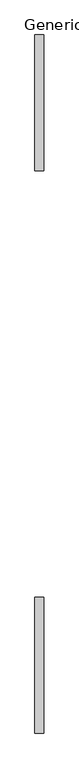
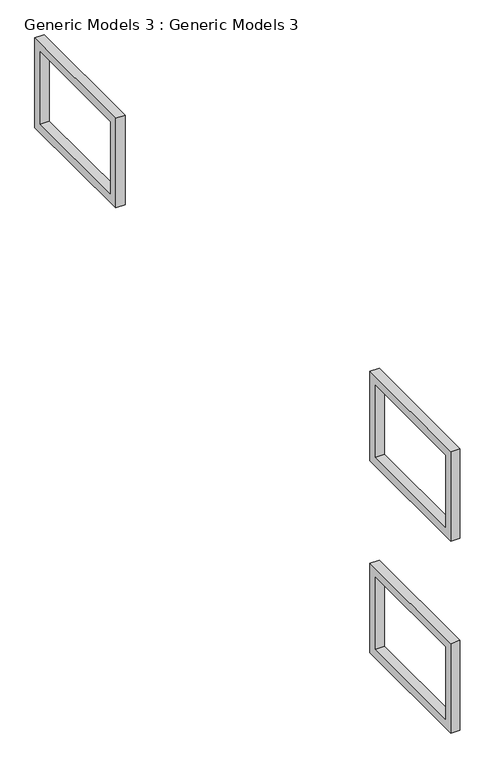
"""IFC4 building model written with IfcOpenShell, lengths in millimetres: proxy geometry, Generic Models 3 : Generic Models 3."""

from ifc_helpers import new_model, si_unit, frame, origin, place, context, project, spatial, polyline, outline, extrude, source, transform, mapped, element, save


def generic_models_3_generic_models_3_62885dc4(model_context):
    return source(origin(), model_context, "Body", "SweptSolid", [
        extrude(outline(polyline([(-2572.1938352, 5765.2), (-257.3938352, 5765.2), (-257.3938352, 4200.4), (-2572.1938352, 4200.4), (-2572.1938352, 5765.2)]), holes=[polyline([(-2419.7938352, 5612.8), (-2419.7938352, 4352.8), (-409.7938352, 4352.8), (-409.7938352, 5612.8), (-2419.7938352, 5612.8)])]), frame((-6909.0474631, 0.0, 0.0), z_axis=(1.0, 0.0, 0.0), x_axis=(0.0, 1.0, 0.0)), (0.0, 0.0, 1.0), 152.4),
        extrude(outline(polyline([(-2572.1938352, 2412.4), (-257.3938352, 2412.4), (-257.3938352, 847.6), (-2572.1938352, 847.6), (-2572.1938352, 2412.4)]), holes=[polyline([(-2419.7938352, 2260.0), (-2419.7938352, 1000.0), (-409.7938352, 1000.0), (-409.7938352, 2260.0), (-2419.7938352, 2260.0)])]), frame((-6909.0474631, 0.0, 0.0), z_axis=(1.0, 0.0, 0.0), x_axis=(0.0, 1.0, 0.0)), (0.0, 0.0, 1.0), 152.4),
        extrude(outline(polyline([(7029.0061648, 5765.2), (9343.8061648, 5765.2), (9343.8061648, 4200.4), (7029.0061648, 4200.4), (7029.0061648, 5765.2)]), holes=[polyline([(7181.4061648, 5612.8), (7181.4061648, 4352.8), (9191.4061648, 4352.8), (9191.4061648, 5612.8), (7181.4061648, 5612.8)])]), frame((-6909.0474631, 0.0, 0.0), z_axis=(1.0, 0.0, 0.0), x_axis=(0.0, 1.0, 0.0)), (0.0, 0.0, 1.0), 152.4),
    ])


if __name__ == "__main__":
    model = new_model("IFC4")
    model_context = context("Model", 3, world=origin())
    ifc_project = project(units=[si_unit("LENGTHUNIT", "METRE", prefix="MILLI")], contexts=[model_context])
    site = spatial("IfcSite", under=ifc_project)
    building = spatial("IfcBuilding", under=site)
    placement = place(None, origin())
    generic_models_3_generic_models_3_shape = generic_models_3_generic_models_3_62885dc4(model_context)
    element("IfcBuildingElementProxy", 1, Name="Generic Models 3 : Generic Models 3", ObjectType="Generic Models 3 : Generic Models 3", at=placement, inside=building, context=model_context, shape_type="MappedRepresentation", body=[
        mapped(generic_models_3_generic_models_3_shape, transform((0.0, 0.0, 0.0), x_axis=(1.0, 0.0, 0.0), y_axis=(0.0, 1.0, 0.0), z_axis=(0.0, 0.0, 1.0))),
    ])
    save(model, "model.ifc")

# Revit data of these elements
# Element 1 (IfcBuildingElementProxy, "Generic Models 3 : Generic Models 3")
#   Materials on its faces: "WALL PAINT"
# Materials
#   "WALL PAINT": class "Generic", colour RGB 120 120 120, transparency 0, Cost = 0
